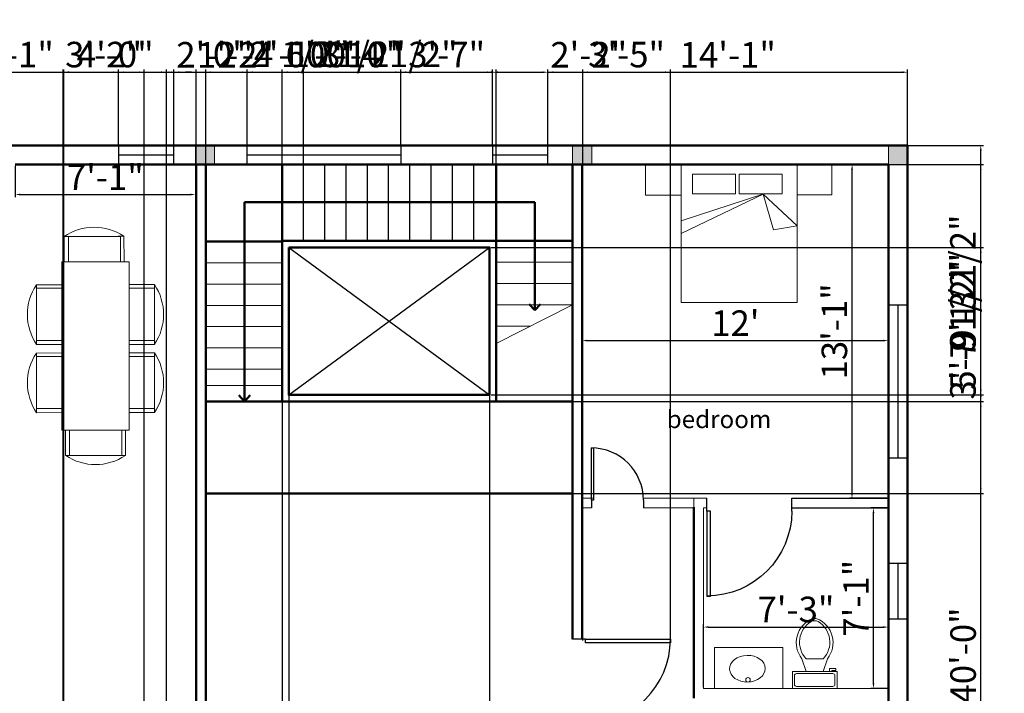
# Model space of a CAD drawing. Units: inches. Extents: x 1367 to 2309, y 1406 to 3826.
# Tile 3 of 9: x 1691 to 2154, y 1853 to 2170. Entities that reach past the tile are written whole.
import ezdxf

# ---------------------------------------------------------------- set-up
doc = ezdxf.new("R2010")
doc.units = ezdxf.units.IN
for name, color, linetype, lineweight in [('A-ANNO-DIMS', 2, 'Continuous', 18), ('A-AREA-IDEN', 3, 'Continuous', 18), ('A-DOOR', 4, 'Continuous', 25), ('A-FLOR-FIXT', 8, 'Continuous', 18), ('A-FLOR-STRS', 7, 'Continuous', 25), ('A-FURN', 8, 'Continuous', 18), ('A-GLAZ', 4, 'Continuous', 25), ('A-WALL', 7, 'Continuous', 50), ('A-WALL-PATT', 8, 'Continuous', 18)]:
    doc.layers.add(name, color=color, linetype=linetype, lineweight=lineweight)
doc.styles.get("Standard").update_dxf_attribs({"font": 'arial.ttf'})
doc.dimstyles.new('ISO-25', dxfattribs={"dimtxt": 12, "dimasz": 2.5, "dimexe": 1.25, "dimexo": 0.625, "dimtad": 1, "dimdec": 0, "dimlunit": 4, "dimtxsty": 'Standard', "dimcen": 2.5, "dimadec": 0, "dimazin": 0, "dimtfac": 1, "dimtdec": 0, "dimtmove": 0, "dimatfit": 3, "dimfxl": 1, "dimarcsym": 0})

# ---------------------------------------------------------------- blocks, each defined once
blk = doc.blocks.new('*U2')
for p, q in [((0, 0), (0, -6)), ((40, 0), (40, -6))]:
    blk.add_line(p, q)
blk.add_lwpolyline([(0, 0), (0, 40), (1.75, 40), (1.75, 0)], close=True)
blk.add_arc((0, 0), 40, 0, 90)
blk = doc.blocks.new('*U4')
for p, q in [((9.5, -6), (9.5, -2)), ((-10, -8.5), (-8, -8.5)), ((-10, -9.5), (-10, -8.5)), ((-8, -8.5), (-8, -8)), ((-7, -8), (-7, -9.5)), ((-4, -8), (-6, -14)), ((4, -8), (6, -14)), ((-7, -9.5), (-10, -9.5)), ((4, -14), (-4, -14))]:
    blk.add_line(p, q)
blk.add_lwpolyline([(10.5, -8), (10.5, 0), (-10.5, 0), (-10.5, -8)], close=True)
for points in [[(-9.5, -2), (-9.5, -6)], [(8.5, -1), (-8.5, -1)], [(-8.5, -7), (8.5, -7)]]:
    blk.add_lwpolyline(points)
for centre, radius, start, end in [((-8.62, -1.88), 0.884, 81.8699, 188.1301), ((8.62, -1.88), 0.884, 351.8699, 98.1301), ((-8.62, -6.12), 0.884, 171.8699, 278.1301), ((8.62, -6.12), 0.884, 261.8699, 8.1301), ((3.52, -21.58), 12.17, 141.4691, 247.9714), ((4.2, -21.82), 11.33, 136.3677, 238.9468), ((-3.52, -21.58), 12.17, 292.0284, 38.5307), ((-4.2, -21.82), 11.33, 301.053, 43.6321), ((0, -27.88), 4, 245.7318, 294.2682), ((0, -29), 4, 254.8605, 285.1395)]:
    blk.add_arc(centre, radius, start, end)
blk = doc.blocks.new('*D27')
at = {"layer": 'A-ANNO-DIMS', "color": 0, "lineweight": -2, "transparency": 16777216}
for p, q in [((1688.87, 2101.5), (1688.87, 2086.74)), ((1773.66, 2101.5), (1773.66, 2086.74)), ((1691.37, 2087.99), (1771.16, 2087.99))]:
    blk.add_line(p, q, dxfattribs=at)
at = {"layer": 'A-ANNO-DIMS', "color": 0, "lineweight": 100, "transparency": 16777216}
for points in [[(1691.37, 2088.41), (1691.37, 2087.58), (1688.87, 2087.99)], [(1771.16, 2088.41), (1771.16, 2087.58), (1773.66, 2087.99)]]:
    blk.add_solid(points, dxfattribs=at)
at = {"layer": 'Defpoints', "color": 0, "lineweight": 100, "transparency": 16777216}
for p in [(1688.87, 2102.13), (1773.66, 2102.13), (1773.66, 2087.99)]:
    blk.add_point(p, dxfattribs=at)
at = {"layer": 'A-ANNO-DIMS', "color": 0, "transparency": 16777216, "insert": (1731.27, 2094.64), "char_height": 12, "attachment_point": 5}
blk.add_mtext('7\'-1"', dxfattribs=at)
blk = doc.blocks.new('*D28')
at = {"layer": 'A-ANNO-DIMS', "color": 0, "lineweight": -2, "transparency": 16777216}
for p, q in [((1955.49, 2101.5), (1955.49, 2018.02)), ((2099.49, 2101.5), (2099.49, 2018.02)), ((1957.99, 2019.27), (2096.99, 2019.27))]:
    blk.add_line(p, q, dxfattribs=at)
at = {"layer": 'A-ANNO-DIMS', "color": 0, "lineweight": 100, "transparency": 16777216}
for points in [[(1957.99, 2019.69), (1957.99, 2018.85), (1955.49, 2019.27)], [(2096.99, 2019.69), (2096.99, 2018.85), (2099.49, 2019.27)]]:
    blk.add_solid(points, dxfattribs=at)
at = {"layer": 'Defpoints', "color": 0, "lineweight": 100, "transparency": 16777216}
for p in [(1955.49, 2102.13), (2099.49, 2102.13), (2099.49, 2019.27)]:
    blk.add_point(p, dxfattribs=at)
at = {"layer": 'A-ANNO-DIMS', "color": 0, "transparency": 16777216, "insert": (2027.49, 2025.92), "char_height": 12, "attachment_point": 5}
blk.add_mtext("12'", dxfattribs=at)
blk = doc.blocks.new('*D29')
at = {"layer": 'A-ANNO-DIMS', "color": 0, "lineweight": -2, "transparency": 16777216}
for p, q in [((2098.9, 2102.13), (2081.16, 2102.13)), ((2082.38, 1947.59), (2082.41, 2099.63)), ((2098.87, 1945.09), (2081.13, 1945.09))]:
    blk.add_line(p, q, dxfattribs=at)
at = {"layer": 'A-ANNO-DIMS', "color": 0, "lineweight": 100, "transparency": 16777216}
for points in [[(2081.99, 2099.63), (2082.83, 2099.63), (2082.41, 2102.13)], [(2081.96, 1947.59), (2082.79, 1947.59), (2082.38, 1945.09)]]:
    blk.add_solid(points, dxfattribs=at)
at = {"layer": 'Defpoints', "color": 0, "lineweight": 100, "transparency": 16777216}
for p in [(2082.41, 2102.13), (2099.53, 2102.13), (2099.49, 1945.09)]:
    blk.add_point(p, dxfattribs=at)
at = {"layer": 'A-ANNO-DIMS', "color": 0, "transparency": 16777216, "insert": (2075.64, 2023.61), "char_height": 12, "attachment_point": 5, "rotation": 89.9877}
blk.add_mtext('13\'-1"', dxfattribs=at)
blk = doc.blocks.new('*D30')
at = {"layer": 'A-ANNO-DIMS', "color": 0, "lineweight": -2, "transparency": 16777216}
for p, q in [((2098.87, 1940.59), (2091.22, 1940.59)), ((2092.47, 1858.08), (2092.47, 1938.09)), ((2098.87, 1855.58), (2091.22, 1855.58))]:
    blk.add_line(p, q, dxfattribs=at)
at = {"layer": 'A-ANNO-DIMS', "color": 0, "lineweight": 100, "transparency": 16777216}
for points in [[(2092.05, 1938.09), (2092.89, 1938.09), (2092.47, 1940.59)], [(2092.05, 1858.08), (2092.89, 1858.08), (2092.47, 1855.58)]]:
    blk.add_solid(points, dxfattribs=at)
at = {"layer": 'Defpoints', "color": 0, "lineweight": 100, "transparency": 16777216}
for p in [(2092.47, 1940.59), (2099.49, 1940.59), (2099.49, 1855.58)]:
    blk.add_point(p, dxfattribs=at)
at = {"layer": 'A-ANNO-DIMS', "color": 0, "transparency": 16777216, "insert": (2085.82, 1898.08), "char_height": 12, "attachment_point": 5, "rotation": 90}
blk.add_mtext('7\'-1"', dxfattribs=at)
blk = doc.blocks.new('*D31')
at = {"layer": 'A-ANNO-DIMS', "color": 0, "lineweight": -2, "transparency": 16777216}
for p, q in [((2012.53, 1856.2), (2012.53, 1885.73)), ((2015.03, 1884.48), (2096.99, 1884.48)), ((2099.49, 1856.2), (2099.49, 1885.73))]:
    blk.add_line(p, q, dxfattribs=at)
at = {"layer": 'A-ANNO-DIMS', "color": 0, "lineweight": 100, "transparency": 16777216}
for points in [[(2015.03, 1884.9), (2015.03, 1884.07), (2012.53, 1884.48)], [(2096.99, 1884.9), (2096.99, 1884.07), (2099.49, 1884.48)]]:
    blk.add_solid(points, dxfattribs=at)
at = {"layer": 'Defpoints', "color": 0, "lineweight": 100, "transparency": 16777216}
for p in [(2099.49, 1884.48), (2012.53, 1855.58), (2099.49, 1855.58)]:
    blk.add_point(p, dxfattribs=at)
at = {"layer": 'A-ANNO-DIMS', "color": 0, "transparency": 16777216, "insert": (2056.01, 1891.24), "char_height": 12, "attachment_point": 5}
blk.add_mtext('7\'-3"', dxfattribs=at)
blk = doc.blocks.new('CHAIR')
for p, q in [((0, 28.09), (11.92, 28.09)), ((11.92, 28.09), (11.92, 24.96)), ((0, 0), (11.92, 0)), ((11.92, 0), (11.92, 2.65))]:
    blk.add_line(p, q)
blk.add_arc((-8.81, 14.05), 25.04, 325.887, 34.113)
blk = doc.blocks.new('*D60')
at = {"layer": 'A-ANNO-DIMS', "color": 0, "lineweight": -2, "transparency": 16777216}
for p, q in [((1640.53, 2111.75), (1640.53, 2146.78)), ((1643.03, 2145.53), (1734.96, 2145.53)), ((1737.46, 2111.75), (1737.46, 2146.78))]:
    blk.add_line(p, q, dxfattribs=at)
at = {"layer": 'A-ANNO-DIMS', "color": 0, "lineweight": 100, "transparency": 16777216}
for points in [[(1643.03, 2145.94), (1643.03, 2145.11), (1640.53, 2145.53)], [(1734.96, 2145.94), (1734.96, 2145.11), (1737.46, 2145.53)]]:
    blk.add_solid(points, dxfattribs=at)
at = {"layer": 'Defpoints', "color": 0, "lineweight": 100, "transparency": 16777216}
for p in [(1737.46, 2145.53), (1640.53, 2111.13), (1737.46, 2111.13)]:
    blk.add_point(p, dxfattribs=at)
at = {"layer": 'A-ANNO-DIMS', "color": 0, "transparency": 16777216, "insert": (1688.99, 2152.28), "char_height": 12, "attachment_point": 5}
blk.add_mtext('8\'-1"', dxfattribs=at)
blk = doc.blocks.new('*D61')
at = {"layer": 'A-ANNO-DIMS', "color": 0, "lineweight": -2, "transparency": 16777216}
for p, q in [((1737.46, 2111.75), (1737.46, 2146.78)), ((1739.96, 2145.53), (1761.02, 2145.53)), ((1763.52, 2111.75), (1763.52, 2146.78)), ((1763.52, 2145.53), (1799.38, 2145.53))]:
    blk.add_line(p, q, dxfattribs=at)
at = {"layer": 'A-ANNO-DIMS', "color": 0, "lineweight": 100, "transparency": 16777216}
for points in [[(1739.96, 2145.94), (1739.96, 2145.11), (1737.46, 2145.53)], [(1761.02, 2145.94), (1761.02, 2145.11), (1763.52, 2145.53)]]:
    blk.add_solid(points, dxfattribs=at)
at = {"layer": 'Defpoints', "color": 0, "lineweight": 100, "transparency": 16777216}
for p in [(1763.52, 2145.53), (1737.46, 2111.13), (1763.52, 2111.13)]:
    blk.add_point(p, dxfattribs=at)
at = {"layer": 'A-ANNO-DIMS', "color": 0, "transparency": 16777216, "insert": (1782.7, 2152.18), "char_height": 12, "attachment_point": 5}
blk.add_mtext('2\'-2"', dxfattribs=at)
blk = doc.blocks.new('*D62')
at = {"layer": 'A-ANNO-DIMS', "color": 0, "lineweight": -2, "transparency": 16777216}
for p, q in [((1763.52, 2111.75), (1763.52, 2146.78)), ((1766.02, 2145.53), (1795.49, 2145.53)), ((1797.99, 2111.75), (1797.99, 2146.78)), ((1797.99, 2145.53), (1871.13, 2145.53))]:
    blk.add_line(p, q, dxfattribs=at)
at = {"layer": 'A-ANNO-DIMS', "color": 0, "lineweight": 100, "transparency": 16777216}
for points in [[(1766.02, 2145.94), (1766.02, 2145.11), (1763.52, 2145.53)], [(1795.49, 2145.94), (1795.49, 2145.11), (1797.99, 2145.53)]]:
    blk.add_solid(points, dxfattribs=at)
at = {"layer": 'Defpoints', "color": 0, "lineweight": 100, "transparency": 16777216}
for p in [(1797.99, 2145.53), (1763.52, 2111.13), (1797.99, 2111.13)]:
    blk.add_point(p, dxfattribs=at)
at = {"layer": 'A-ANNO-DIMS', "color": 0, "transparency": 16777216, "insert": (1835.81, 2152.36), "char_height": 12, "attachment_point": 5}
blk.add_mtext('2\'-10 1/2"', dxfattribs=at)
blk = doc.blocks.new('*D63')
at = {"layer": 'A-ANNO-DIMS', "color": 0, "lineweight": -2, "transparency": 16777216}
for p, q in [((1797.99, 2111.75), (1797.99, 2146.78)), ((1800.49, 2145.53), (1867.65, 2145.53)), ((1870.15, 2111.75), (1870.15, 2146.78))]:
    blk.add_line(p, q, dxfattribs=at)
at = {"layer": 'A-ANNO-DIMS', "color": 0, "lineweight": 100, "transparency": 16777216}
for points in [[(1800.49, 2145.94), (1800.49, 2145.11), (1797.99, 2145.53)], [(1867.65, 2145.94), (1867.65, 2145.11), (1870.15, 2145.53)]]:
    blk.add_solid(points, dxfattribs=at)
at = {"layer": 'Defpoints', "color": 0, "lineweight": 100, "transparency": 16777216}
for p in [(1870.15, 2145.53), (1797.99, 2111.13), (1870.15, 2111.13)]:
    blk.add_point(p, dxfattribs=at)
at = {"layer": 'A-ANNO-DIMS', "color": 0, "transparency": 16777216, "insert": (1834.07, 2152.28), "char_height": 12, "attachment_point": 5}
blk.add_mtext('6\'-0"', dxfattribs=at)
blk = doc.blocks.new('*D64')
at = {"layer": 'A-ANNO-DIMS', "color": 0, "lineweight": -2, "transparency": 16777216}
for p, q in [((1870.15, 2111.75), (1870.15, 2146.78)), ((1872.65, 2145.53), (1910.84, 2145.53)), ((1913.34, 2111.75), (1913.34, 2146.78))]:
    blk.add_line(p, q, dxfattribs=at)
at = {"layer": 'A-ANNO-DIMS', "color": 0, "lineweight": 100, "transparency": 16777216}
for points in [[(1872.65, 2145.94), (1872.65, 2145.11), (1870.15, 2145.53)], [(1910.84, 2145.94), (1910.84, 2145.11), (1913.34, 2145.53)]]:
    blk.add_solid(points, dxfattribs=at)
at = {"layer": 'Defpoints', "color": 0, "lineweight": 100, "transparency": 16777216}
for p in [(1913.34, 2145.53), (1870.15, 2111.13), (1913.34, 2111.13)]:
    blk.add_point(p, dxfattribs=at)
at = {"layer": 'A-ANNO-DIMS', "color": 0, "transparency": 16777216, "insert": (1891.75, 2152.28), "char_height": 12, "attachment_point": 5}
blk.add_mtext('3\'-7"', dxfattribs=at)
blk = doc.blocks.new('*D65')
at = {"layer": 'A-ANNO-DIMS', "color": 0, "lineweight": -2, "transparency": 16777216}
for p, q in [((1913.34, 2111.75), (1913.34, 2146.78)), ((1915.84, 2145.53), (1936.9, 2145.53)), ((1939.4, 2111.75), (1939.4, 2146.78)), ((1939.4, 2145.53), (1975.25, 2145.53))]:
    blk.add_line(p, q, dxfattribs=at)
at = {"layer": 'A-ANNO-DIMS', "color": 0, "lineweight": 100, "transparency": 16777216}
for points in [[(1915.84, 2145.94), (1915.84, 2145.11), (1913.34, 2145.53)], [(1936.9, 2145.94), (1936.9, 2145.11), (1939.4, 2145.53)]]:
    blk.add_solid(points, dxfattribs=at)
at = {"layer": 'Defpoints', "color": 0, "lineweight": 100, "transparency": 16777216}
for p in [(1939.4, 2145.53), (1913.34, 2111.13), (1939.4, 2111.13)]:
    blk.add_point(p, dxfattribs=at)
at = {"layer": 'A-ANNO-DIMS', "color": 0, "transparency": 16777216, "insert": (1958.58, 2152.18), "char_height": 12, "attachment_point": 5}
blk.add_mtext('2\'-2"', dxfattribs=at)
blk = doc.blocks.new('*D66')
at = {"layer": 'A-ANNO-DIMS', "color": 0, "lineweight": -2, "transparency": 16777216}
for p, q in [((1939.4, 2111.75), (1939.4, 2146.78)), ((1941.9, 2145.53), (2106.03, 2145.53)), ((2108.53, 2111.75), (2108.53, 2146.78))]:
    blk.add_line(p, q, dxfattribs=at)
at = {"layer": 'A-ANNO-DIMS', "color": 0, "lineweight": 100, "transparency": 16777216}
for points in [[(1941.9, 2145.94), (1941.9, 2145.11), (1939.4, 2145.53)], [(2106.03, 2145.94), (2106.03, 2145.11), (2108.53, 2145.53)]]:
    blk.add_solid(points, dxfattribs=at)
at = {"layer": 'Defpoints', "color": 0, "lineweight": 100, "transparency": 16777216}
for p in [(2108.53, 2145.53), (1939.4, 2111.13), (2108.53, 2111.13)]:
    blk.add_point(p, dxfattribs=at)
at = {"layer": 'A-ANNO-DIMS', "color": 0, "transparency": 16777216, "insert": (2023.96, 2152.18), "char_height": 12, "attachment_point": 5}
blk.add_mtext('14\'-1"', dxfattribs=at)
blk = doc.blocks.new('*D67')
at = {"layer": 'A-ANNO-DIMS', "color": 0, "lineweight": -2, "transparency": 16777216}
for p, q in [((2109.15, 2111.13), (2144.18, 2111.13)), ((2142.93, 1633.63), (2142.93, 2108.63)), ((2109.12, 1631.13), (2144.18, 1631.13))]:
    blk.add_line(p, q, dxfattribs=at)
at = {"layer": 'A-ANNO-DIMS', "color": 0, "lineweight": 100, "transparency": 16777216}
for points in [[(2142.51, 2108.63), (2143.34, 2108.63), (2142.93, 2111.13)], [(2142.51, 1633.63), (2143.34, 1633.63), (2142.93, 1631.13)]]:
    blk.add_solid(points, dxfattribs=at)
at = {"layer": 'Defpoints', "color": 0, "lineweight": 100, "transparency": 16777216}
for p in [(2108.53, 2111.13), (2142.93, 2111.13), (2108.49, 1631.13)]:
    blk.add_point(p, dxfattribs=at)
at = {"layer": 'A-ANNO-DIMS', "color": 0, "transparency": 16777216, "insert": (2136.17, 1871.13), "char_height": 12, "attachment_point": 5, "rotation": 90}
blk.add_mtext('40\'-0"', dxfattribs=at)
blk = doc.blocks.new('*D76')
at = {"layer": 'A-ANNO-DIMS', "color": 0, "lineweight": -2, "transparency": 16777216}
for p, q in [((1711.82, 1517.28), (1711.82, 2146.78)), ((1714.32, 2145.53), (1757.51, 2145.53)), ((1760.01, 1517.28), (1760.01, 2146.78))]:
    blk.add_line(p, q, dxfattribs=at)
at = {"layer": 'A-ANNO-DIMS', "color": 0, "lineweight": 100, "transparency": 16777216}
for points in [[(1714.32, 2145.94), (1714.32, 2145.11), (1711.82, 2145.53)], [(1757.51, 2145.94), (1757.51, 2145.11), (1760.01, 2145.53)]]:
    blk.add_solid(points, dxfattribs=at)
at = {"layer": 'Defpoints', "color": 0, "lineweight": 100, "transparency": 16777216}
for p in [(1760.01, 2145.53), (1711.82, 1516.65), (1760.01, 1516.65)]:
    blk.add_point(p, dxfattribs=at)
at = {"layer": 'A-ANNO-DIMS', "color": 0, "transparency": 16777216, "insert": (1735.92, 2152.28), "char_height": 12, "attachment_point": 5}
blk.add_mtext('4\'-0"', dxfattribs=at)
blk = doc.blocks.new('*D77')
at = {"layer": 'A-ANNO-DIMS', "color": 0, "lineweight": -2, "transparency": 16777216}
for p, q in [((1760.01, 1493.18), (1760.01, 2146.78)), ((1762.51, 2145.53), (1771.49, 2145.53)), ((1773.99, 1493.56), (1773.99, 2146.78)), ((1773.99, 2145.53), (1808.51, 2145.53))]:
    blk.add_line(p, q, dxfattribs=at)
at = {"layer": 'A-ANNO-DIMS', "color": 0, "lineweight": 100, "transparency": 16777216}
for points in [[(1762.51, 2145.94), (1762.51, 2145.11), (1760.01, 2145.53)], [(1771.49, 2145.94), (1771.49, 2145.11), (1773.99, 2145.53)]]:
    blk.add_solid(points, dxfattribs=at)
at = {"layer": 'Defpoints', "color": 0, "lineweight": 100, "transparency": 16777216}
for p in [(1773.99, 2145.53), (1760.01, 1492.55), (1773.99, 1492.94)]:
    blk.add_point(p, dxfattribs=at)
at = {"layer": 'A-ANNO-DIMS', "color": 0, "transparency": 16777216, "insert": (1792.5, 2152.18), "char_height": 12, "attachment_point": 5}
blk.add_mtext('1\'-2"', dxfattribs=at)
blk = doc.blocks.new('*D78')
at = {"layer": 'A-ANNO-DIMS', "color": 0, "lineweight": -2, "transparency": 16777216}
for p, q in [((1711.4, 1640.75), (1711.4, 2146.78)), ((1713.9, 2145.53), (1747.03, 2145.53)), ((1749.53, 1640.75), (1749.53, 2146.78))]:
    blk.add_line(p, q, dxfattribs=at)
at = {"layer": 'A-ANNO-DIMS', "color": 0, "lineweight": 100, "transparency": 16777216}
for points in [[(1713.9, 2145.94), (1713.9, 2145.11), (1711.4, 2145.53)], [(1747.03, 2145.94), (1747.03, 2145.11), (1749.53, 2145.53)]]:
    blk.add_solid(points, dxfattribs=at)
at = {"layer": 'Defpoints', "color": 0, "lineweight": 100, "transparency": 16777216}
for p in [(1749.53, 2145.53), (1711.4, 1640.13), (1749.53, 1640.13)]:
    blk.add_point(p, dxfattribs=at)
at = {"layer": 'A-ANNO-DIMS', "color": 0, "transparency": 16777216, "insert": (1730.47, 2152.28), "char_height": 12, "attachment_point": 5}
blk.add_mtext('3\'-2"', dxfattribs=at)
blk = doc.blocks.new('*D79')
at = {"layer": 'A-ANNO-DIMS', "color": 0, "lineweight": -2, "transparency": 16777216}
for p, q in [((1778.49, 1990.06), (1778.49, 1415.33)), ((1814.49, 1990.06), (1814.49, 1415.33)), ((1780.99, 1416.58), (1811.99, 1416.58))]:
    blk.add_line(p, q, dxfattribs=at)
at = {"layer": 'A-ANNO-DIMS', "color": 0, "lineweight": 100, "transparency": 16777216}
for points in [[(1780.99, 1416.99), (1780.99, 1416.16), (1778.49, 1416.58)], [(1811.99, 1416.99), (1811.99, 1416.16), (1814.49, 1416.58)]]:
    blk.add_solid(points, dxfattribs=at)
at = {"layer": 'Defpoints', "color": 0, "lineweight": 100, "transparency": 16777216}
for p in [(1778.49, 1990.68), (1814.49, 1990.68), (1814.49, 1416.58)]:
    blk.add_point(p, dxfattribs=at)
at = {"layer": 'A-ANNO-DIMS', "color": 0, "transparency": 16777216, "insert": (1796.49, 1423.33), "char_height": 12, "attachment_point": 5}
blk.add_mtext('3\'-0"', dxfattribs=at)
blk = doc.blocks.new('*D80')
at = {"layer": 'A-ANNO-DIMS', "color": 0, "lineweight": -2, "transparency": 16777216}
for p, q in [((1817.49, 1993.06), (1817.49, 1415.33)), ((1911.99, 1993.06), (1911.99, 1415.33)), ((1819.99, 1416.58), (1909.49, 1416.58))]:
    blk.add_line(p, q, dxfattribs=at)
at = {"layer": 'A-ANNO-DIMS', "color": 0, "lineweight": 100, "transparency": 16777216}
for points in [[(1819.99, 1416.99), (1819.99, 1416.16), (1817.49, 1416.58)], [(1909.49, 1416.99), (1909.49, 1416.16), (1911.99, 1416.58)]]:
    blk.add_solid(points, dxfattribs=at)
at = {"layer": 'Defpoints', "color": 0, "lineweight": 100, "transparency": 16777216}
for p in [(1817.49, 1993.68), (1911.99, 1993.68), (1911.99, 1416.58)]:
    blk.add_point(p, dxfattribs=at)
at = {"layer": 'A-ANNO-DIMS', "color": 0, "transparency": 16777216, "insert": (1864.74, 1423.41), "char_height": 12, "attachment_point": 5}
blk.add_mtext('7\'-10 1/2"', dxfattribs=at)
blk = doc.blocks.new('*D81')
at = {"layer": 'A-ANNO-DIMS', "color": 0, "lineweight": -2, "transparency": 16777216}
for p, q in [((1912.62, 2063.13), (2144.18, 2063.13)), ((2142.93, 1996.18), (2142.93, 2060.63)), ((1912.62, 1993.68), (2144.18, 1993.68))]:
    blk.add_line(p, q, dxfattribs=at)
at = {"layer": 'A-ANNO-DIMS', "color": 0, "lineweight": 100, "transparency": 16777216}
for points in [[(2142.51, 2060.63), (2143.34, 2060.63), (2142.93, 2063.13)], [(2142.51, 1996.18), (2143.34, 1996.18), (2142.93, 1993.68)]]:
    blk.add_solid(points, dxfattribs=at)
at = {"layer": 'Defpoints', "color": 0, "lineweight": 100, "transparency": 16777216}
for p in [(1911.99, 2063.13), (2142.93, 2063.13), (1911.99, 1993.68)]:
    blk.add_point(p, dxfattribs=at)
at = {"layer": 'A-ANNO-DIMS', "color": 0, "transparency": 16777216, "insert": (2136.1, 2028.41), "char_height": 12, "attachment_point": 5, "rotation": 90}
blk.add_mtext('5\'-9 1/2"', dxfattribs=at)
blk = doc.blocks.new('*D82')
at = {"layer": 'A-ANNO-DIMS', "color": 0, "lineweight": -2, "transparency": 16777216}
for p, q in [((1814.49, 2066.46), (1814.49, 2146.78)), ((1816.99, 2145.53), (1912.49, 2145.53)), ((1914.99, 2066.75), (1914.99, 2146.78))]:
    blk.add_line(p, q, dxfattribs=at)
at = {"layer": 'A-ANNO-DIMS', "color": 0, "lineweight": 100, "transparency": 16777216}
for points in [[(1816.99, 2145.94), (1816.99, 2145.11), (1814.49, 2145.53)], [(1912.49, 2145.94), (1912.49, 2145.11), (1914.99, 2145.53)]]:
    blk.add_solid(points, dxfattribs=at)
at = {"layer": 'Defpoints', "color": 0, "lineweight": 100, "transparency": 16777216}
for p in [(1914.99, 2145.53), (1814.49, 2065.83), (1914.99, 2066.13)]:
    blk.add_point(p, dxfattribs=at)
at = {"layer": 'A-ANNO-DIMS', "color": 0, "transparency": 16777216, "insert": (1864.74, 2152.36), "char_height": 12, "attachment_point": 5}
blk.add_mtext('8\'-4 1/2"', dxfattribs=at)
blk = doc.blocks.new('*D83')
at = {"layer": 'A-ANNO-DIMS', "color": 0, "lineweight": -2, "transparency": 16777216}
for p, q in [((1814.49, 2066.46), (1814.49, 2146.78)), ((1816.99, 2145.53), (1821.99, 2145.53)), ((1824.49, 2066.46), (1824.49, 2146.78)), ((1824.49, 2145.53), (1869.47, 2145.53))]:
    blk.add_line(p, q, dxfattribs=at)
at = {"layer": 'A-ANNO-DIMS', "color": 0, "lineweight": 100, "transparency": 16777216}
for points in [[(1816.99, 2145.94), (1816.99, 2145.11), (1814.49, 2145.53)], [(1821.99, 2145.94), (1821.99, 2145.11), (1824.49, 2145.53)]]:
    blk.add_solid(points, dxfattribs=at)
at = {"layer": 'Defpoints', "color": 0, "lineweight": 100, "transparency": 16777216}
for p in [(1824.49, 2145.53), (1814.49, 2065.83), (1824.49, 2065.83)]:
    blk.add_point(p, dxfattribs=at)
at = {"layer": 'A-ANNO-DIMS', "color": 0, "transparency": 16777216, "insert": (1848.23, 2152.28), "char_height": 12, "attachment_point": 5}
blk.add_mtext('0\'-10"', dxfattribs=at)
blk = doc.blocks.new('*D84')
at = {"layer": 'A-ANNO-DIMS', "color": 0, "lineweight": -2, "transparency": 16777216}
for p, q in [((2142.93, 1990.68), (2142.93, 2054.29)), ((1951.62, 1990.68), (2144.18, 1990.68)), ((2142.93, 1949.83), (2142.93, 1988.18)), ((1951.62, 1947.33), (2144.18, 1947.33))]:
    blk.add_line(p, q, dxfattribs=at)
at = {"layer": 'A-ANNO-DIMS', "color": 0, "lineweight": 100, "transparency": 16777216}
for points in [[(2142.51, 1988.18), (2143.34, 1988.18), (2142.93, 1990.68)], [(2142.51, 1949.83), (2143.34, 1949.83), (2142.93, 1947.33)]]:
    blk.add_solid(points, dxfattribs=at)
at = {"layer": 'Defpoints', "color": 0, "lineweight": 100, "transparency": 16777216}
for p in [(1950.99, 1990.68), (2142.93, 1990.68), (1950.99, 1947.33)]:
    blk.add_point(p, dxfattribs=at)
at = {"layer": 'A-ANNO-DIMS', "color": 0, "transparency": 16777216, "insert": (2136.09, 2023.73), "char_height": 12, "attachment_point": 5, "rotation": 90}
blk.add_mtext('3\'-7 1/2"', dxfattribs=at)
blk = doc.blocks.new('*D85')
at = {"layer": 'A-ANNO-DIMS', "color": 0, "lineweight": -2, "transparency": 16777216}
for p, q in [((1951.62, 2102.13), (2144.18, 2102.13)), ((2142.93, 1993.18), (2142.93, 2099.63)), ((1951.62, 1990.68), (2144.18, 1990.68))]:
    blk.add_line(p, q, dxfattribs=at)
at = {"layer": 'A-ANNO-DIMS', "color": 0, "lineweight": 100, "transparency": 16777216}
for points in [[(2142.51, 2099.63), (2143.34, 2099.63), (2142.93, 2102.13)], [(2142.51, 1993.18), (2143.34, 1993.18), (2142.93, 1990.68)]]:
    blk.add_solid(points, dxfattribs=at)
at = {"layer": 'Defpoints', "color": 0, "lineweight": 100, "transparency": 16777216}
for p in [(1950.99, 2102.13), (2142.93, 2102.13), (1950.99, 1990.68)]:
    blk.add_point(p, dxfattribs=at)
at = {"layer": 'A-ANNO-DIMS', "color": 0, "transparency": 16777216, "insert": (2136.09, 2046.41), "char_height": 12, "attachment_point": 5, "rotation": 90}
blk.add_mtext('9\'-3 1/2"', dxfattribs=at)
blk = doc.blocks.new('*D86')
at = {"layer": 'A-ANNO-DIMS', "color": 0, "lineweight": -2, "transparency": 16777216}
for p, q in [((1771.49, 2145.53), (1768.99, 2145.53)), ((1773.99, 2102.75), (1773.99, 2146.78)), ((1773.99, 2145.53), (1778.49, 2145.53)), ((1778.49, 2102.75), (1778.49, 2146.78)), ((1780.99, 2145.53), (1844.6, 2145.53))]:
    blk.add_line(p, q, dxfattribs=at)
at = {"layer": 'A-ANNO-DIMS', "color": 0, "lineweight": 100, "transparency": 16777216}
for points in [[(1771.49, 2145.94), (1771.49, 2145.11), (1773.99, 2145.53)], [(1780.99, 2145.94), (1780.99, 2145.11), (1778.49, 2145.53)]]:
    blk.add_solid(points, dxfattribs=at)
at = {"layer": 'Defpoints', "color": 0, "lineweight": 100, "transparency": 16777216}
for p in [(1778.49, 2145.53), (1773.99, 2102.13), (1778.49, 2102.13)]:
    blk.add_point(p, dxfattribs=at)
at = {"layer": 'A-ANNO-DIMS', "color": 0, "transparency": 16777216, "insert": (1814.05, 2152.36), "char_height": 12, "attachment_point": 5}
blk.add_mtext('0\'-4 1/2"', dxfattribs=at)
blk = doc.blocks.new('*D137')
at = {"layer": 'A-ANNO-DIMS', "color": 0, "lineweight": -2, "transparency": 16777216}
for p, q in [((1955.76, 1878.24), (1955.76, 2146.78)), ((1958.26, 2145.53), (1994.49, 2145.53)), ((1996.99, 1877.73), (1996.99, 2146.78))]:
    blk.add_line(p, q, dxfattribs=at)
at = {"layer": 'A-ANNO-DIMS', "color": 0, "lineweight": 100, "transparency": 16777216}
for points in [[(1958.26, 2145.94), (1958.26, 2145.11), (1955.76, 2145.53)], [(1994.49, 2145.94), (1994.49, 2145.11), (1996.99, 2145.53)]]:
    blk.add_solid(points, dxfattribs=at)
at = {"layer": 'Defpoints', "color": 0, "lineweight": 100, "transparency": 16777216}
for p in [(1996.99, 2145.53), (1955.76, 1877.62), (1996.99, 1877.1)]:
    blk.add_point(p, dxfattribs=at)
at = {"layer": 'A-ANNO-DIMS', "color": 0, "transparency": 16777216, "insert": (1976.37, 2152.28), "char_height": 12, "attachment_point": 5}
blk.add_mtext('3\'-5"', dxfattribs=at)

msp = doc.modelspace()

# ---------------------------------------------------------------- hatches: boundary and pattern name
at = {"layer": 'A-WALL-PATT'}
h = msp.add_hatch(color=256, dxfattribs=at)
h.dxf.hatch_style = 1
h.paths.add_polyline_path([(2108.49, 2102.13), (2108.49, 2111.13), (2099.53, 2111.13), (2099.53, 2102.13)])
h.paths.add_polyline_path([(1959.99, 2102.13), (1959.99, 2111.13), (1950.99, 2111.13), (1950.99, 2102.13)])
h.paths.add_polyline_path([(1773.66, 2111.13), (1773.66, 2102.13), (1782.66, 2102.13), (1782.66, 2111.13)])
h = msp.add_hatch(color=256, dxfattribs=at)
h.dxf.hatch_style = 1
h.paths.add_polyline_path([(1508.49, 1631.13), (1517.49, 1631.13), (1517.49, 1640.13), (1508.49, 1640.13)])
h.paths.add_polyline_path([(1773.99, 1631.13), (1782.99, 1631.13), (1782.99, 1640.13), (1773.99, 1640.13)])
h.paths.add_polyline_path([(1959.99, 1631.13), (1959.99, 1640.13), (1950.99, 1640.13), (1950.99, 1631.13)])
h.paths.add_polyline_path([(2099.49, 1640.13), (2099.49, 1631.13), (2108.49, 1631.13), (2108.49, 1640.13)])
h.paths.add_polyline_path([(1706.06, 1795.81), (1771.22, 1795.81), (1771.22, 1813.02), (1706.06, 1813.02)], flags=9)
h.paths.add_polyline_path([(1573.51, 1725.43), (1623.74, 1725.43), (1623.74, 1742.65), (1573.51, 1742.65)], flags=9)
h.paths.add_polyline_path([(1582.26, 2004.3), (1623.41, 2004.3), (1623.41, 2021.52), (1582.26, 2021.52)], flags=9)
h.paths.add_polyline_path([(1992.39, 1973.53), (2042.62, 1973.53), (2042.62, 1990.75), (1992.39, 1990.75)], flags=9)
h.paths.add_polyline_path([(2015.09, 1737.31), (2065.32, 1737.31), (2065.32, 1754.53), (2015.09, 1754.53)], flags=9)
h.paths.add_polyline_path([(1827.45, 1770.85), (1884.81, 1770.85), (1884.81, 1788.06), (1827.45, 1788.06)], flags=9)

# ---------------------------------------------------------------- linework, layer by layer
at = {"layer": 'A-FLOR-STRS'}
for p, q in [((1824.49, 2065.83), (1824.49, 2102.13)), ((1834.49, 2065.83), (1834.49, 2102.13)), ((1844.49, 2065.83), (1844.49, 2102.13)), ((1854.49, 2065.83), (1854.49, 2102.13)), ((1864.49, 2065.83), (1864.49, 2102.13)), ((1874.49, 2065.83), (1874.49, 2102.13)), ((1884.49, 2065.83), (1884.49, 2102.13)), ((1894.49, 2065.83), (1894.49, 2102.13)), ((1904.49, 2065.83), (1904.49, 2102.13)), ((1817.49, 2063.13), (1911.99, 1993.68)), ((1817.49, 1993.68), (1911.99, 2063.13))]:
    msp.add_line(p, q, dxfattribs=at)
at = {"layer": 'A-FURN'}
for p, q in [((2040.89, 2088.29), (2002.08, 2075.58)), ((2040.89, 2088.29), (2002.08, 2069.66)), ((2040.56, 2088.13), (2056.63, 2073.27)), ((2045.41, 2071.32), (2040.56, 2088.13)), ((2056.63, 2073.27), (2045.41, 2071.32)), ((1778.49, 2055.83), (1814.49, 2055.83)), ((1914.99, 2056.13), (1950.99, 2056.13)), ((1778.49, 2045.83), (1814.49, 2045.83)), ((1914.99, 2046.13), (1950.99, 2046.13)), ((1778.49, 2035.83), (1814.49, 2035.83)), ((1914.99, 2036.13), (1950.99, 2036.13)), ((1914.99, 2017.94), (1950.99, 2036.13)), ((1778.49, 2025.83), (1814.49, 2025.83)), ((1914.99, 2026.13), (1931.19, 2026.13)), ((1778.49, 2015.83), (1814.49, 2015.83)), ((1778.49, 2005.83), (1814.49, 2005.83)), ((1778.49, 1998.12), (1814.49, 1998.12)), ((1960.87, 1945.09), (1955.49, 1945.09)), ((2008.03, 1945.09), (1984.28, 1945.09)), ((2008.03, 1945.09), (2014.06, 1945.09)), ((2008.03, 1940.59), (2008.03, 1945.09)), ((1959.8, 1940.59), (1955.49, 1940.59)), ((2008.03, 1940.59), (1984.29, 1940.59)), ((2004.29, 1940.59), (2008.03, 1940.59)), ((2012.53, 1940.59), (2014.06, 1940.59)), ((2012.53, 1940.59), (2012.53, 1855.58)), ((2017.75, 1855.58), (2017.75, 1874.93)), ((2096.58, 1855.58), (2012.53, 1855.58)), ((2012.53, 1855.58), (2099.49, 1855.58)), ((2096.58, 1855.58), (2099.49, 1855.58))]:
    msp.add_line(p, q, dxfattribs=at)
for points in [[(1773.66, 2111.13), (1782.66, 2111.13), (1782.66, 2102.13), (1773.66, 2102.13)], [(1950.99, 2111.13), (1959.99, 2111.13), (1959.99, 2102.13), (1950.99, 2102.13)], [(2099.53, 2111.13), (2108.53, 2111.13), (2108.53, 2102.13), (2099.53, 2102.13)], [(2002.08, 2102.13), (1985.26, 2102.13), (1985.26, 2087.72), (2002.08, 2087.72)], [(2002.08, 2102.13), (2056.63, 2102.13), (2056.63, 2037.19), (2002.08, 2037.19)], [(2056.63, 2102.13), (2072.9, 2102.13), (2072.9, 2087.87), (2056.63, 2087.87)], [(2007.44, 2097.5), (2027.64, 2097.5), (2027.64, 2088.29), (2007.44, 2088.29)], [(2029.32, 2097.5), (2049.51, 2097.5), (2049.51, 2088.29), (2029.32, 2088.29)], [(1738.42, 2056.37), (1738.42, 2068.29), (1713.9, 2068.29), (1713.9, 2056.37)], [(1710.82, 2056.37), (1742.44, 2056.37), (1742.44, 1977.17), (1710.82, 1977.17)], [(1710.82, 2043.91), (1698.9, 2043.91), (1698.9, 2019.39), (1710.82, 2019.39)], [(1742.44, 2043.91), (1754.36, 2043.91), (1754.36, 2019.39), (1742.44, 2019.39)], [(1710.82, 2011.81), (1698.9, 2011.81), (1698.9, 1987.3), (1710.82, 1987.3)], [(1742.44, 2011.81), (1754.36, 2011.81), (1754.36, 1987.3), (1742.44, 1987.3)], [(1739.01, 1977.17), (1739.01, 1965.25), (1714.49, 1965.25), (1714.49, 1977.17)], [(2017.75, 1874.93), (2017.75, 1855.58), (2049.92, 1855.58), (2049.92, 1874.93)]]:
    msp.add_lwpolyline(points, close=True, dxfattribs=at)
msp.add_circle((2033.44, 1859.68), 1.06, dxfattribs=at)
msp.add_ellipse((2033.19, 1864.89), major_axis=(8.38, 0.17), ratio=0.747916, dxfattribs=at)
at = {"layer": 'A-GLAZ'}
for p, q in [((1737.46, 2106.63), (1763.52, 2106.63)), ((1797.99, 2106.63), (1870.15, 2106.63)), ((1913.34, 2106.63), (1939.4, 2106.63)), ((2103.99, 2036.08), (2103.99, 1963.92)), ((2054.06, 1945.09), (2099.49, 1945.09)), ((2054.06, 1940.59), (2099.49, 1940.59)), ((2103.99, 1914.39), (2103.99, 1888.32))]:
    msp.add_line(p, q, dxfattribs=at)
for points in [[(1737.46, 2102.13), (1763.52, 2102.13), (1763.52, 2111.13), (1737.46, 2111.13)], [(1797.99, 2111.13), (1870.15, 2111.13), (1870.15, 2102.13), (1797.99, 2102.13)], [(1913.34, 2102.13), (1939.4, 2102.13), (1939.4, 2111.13), (1913.34, 2111.13)], [(2108.49, 2036.08), (2108.49, 1963.92), (2099.49, 1963.92), (2099.49, 2036.08)], [(2099.49, 1914.39), (2099.49, 1888.32), (2108.49, 1888.32), (2108.49, 1914.39)]]:
    msp.add_lwpolyline(points, close=True, dxfattribs=at)
at = {"layer": 'A-WALL'}
for p, q in [((1688.87, 2102.13), (1746.15, 2102.13)), ((1773.99, 1947.33), (1773.99, 2102.13)), ((1778.49, 1947.33), (1778.49, 2102.13)), ((1814.49, 2065.83), (1814.49, 2102.13)), ((1896.39, 2102.13), (1848.39, 2102.13)), ((2085.87, 2102.13), (1896.39, 2102.13)), ((1950.99, 2102.13), (1902.99, 2102.13)), ((1950.99, 2102.13), (1902.99, 2102.13)), ((1914.99, 2066.13), (1914.99, 2102.13)), ((1950.99, 2102.13), (1950.99, 1947.33)), ((1950.99, 2102.13), (1950.99, 2066.13)), ((1955.49, 2102.13), (1955.49, 1947.33)), ((2099.49, 2102.13), (1979.49, 2102.13)), ((1796.72, 1990.68), (1796.72, 2084.33)), ((1796.72, 2084.33), (1933.25, 2084.33)), ((1933.25, 2084.33), (1933.25, 2033.57)), ((1778.49, 2065.83), (1814.49, 2065.83)), ((1814.49, 1990.68), (1814.49, 2066.13)), ((1914.99, 2066.13), (1814.49, 2066.13)), ((1914.99, 2066.13), (1914.99, 1990.68)), ((1914.99, 2066.13), (1950.99, 2066.13)), ((1933.25, 2033.57), (1930.64, 2036.48)), ((1933.25, 2033.57), (1935.85, 2036.48)), ((1796.72, 1990.68), (1794.11, 1993.59)), ((1796.72, 1990.68), (1799.33, 1993.59)), ((1778.49, 1990.68), (1950.99, 1990.68)), ((1773.99, 1759.12), (1773.99, 1947.33)), ((1778.49, 1947.33), (1950.99, 1947.33)), ((1778.49, 1759.12), (1778.49, 1947.33)), ((1950.99, 1878.85), (1950.99, 1947.33)), ((1955.49, 1878.85), (1955.49, 1947.33)), ((2008.03, 1940.98), (2008.03, 1855.58)), ((2008.03, 1855.58), (2008.03, 1851.08))]:
    msp.add_line(p, q, dxfattribs=at)
for points in [[(1751.28, 1631.13), (2108.49, 1631.13), (2108.49, 2111.13), (1508.49, 2111.13), (1508.49, 1631.13), (1711.28, 1631.13)], [(2099.49, 1808.62), (2099.49, 2102.13), (1688.87, 2102.13)]]:
    msp.add_lwpolyline(points, dxfattribs=at)
for points in [[(1814.49, 2066.13), (1914.99, 2066.13), (1914.99, 1990.68), (1814.49, 1990.68)], [(1817.49, 2063.13), (1911.99, 2063.13), (1911.99, 1993.68), (1817.49, 1993.68)]]:
    msp.add_lwpolyline(points, close=True, dxfattribs=at)

# ---------------------------------------------------------------- block references
at = {"layer": 'A-DOOR', "xscale": 0.6122238826041507, "yscale": 0.6122238826041507, "zscale": 0.6122238826041507}
msp.add_blockref('*U2', (1959.8, 1944.26), dxfattribs=at)
at = {"layer": 'A-DOOR', "xscale": -1, "rotation": 180}
msp.add_blockref('*U2', (2014.06, 1939.09), dxfattribs=at)
at = {"layer": 'A-DOOR', "rotation": 270}
msp.add_blockref('*U2', (1956.99, 1878.85), dxfattribs=at)
at = {"layer": 'A-FLOR-FIXT', "rotation": 180}
msp.add_blockref('*U4', (2064.82, 1855.58), dxfattribs=at)
at = {"layer": 'A-FURN'}
for p, rotation in [((1740.06, 2056.44), 90.30251730046201), ((1710.75, 2045.55), 180.302517300463), ((1710.75, 2013.46), 180.3025173004606), ((1712.61, 1977.17), 270.0000000000039)]:
    msp.add_blockref('CHAIR', p, dxfattribs=dict(at, rotation=rotation))
for p in [(1742.44, 2017.51), (1742.44, 1985.42)]:
    msp.add_blockref('CHAIR', p, dxfattribs=at)

# ---------------------------------------------------------------- texts
at = {"layer": 'A-AREA-IDEN', "insert": (1995.24, 1986.45), "char_height": 8.353, "attachment_point": 1}
msp.add_mtext_dynamic_manual_height_columns('bedroom', width=204.251, gutter_width=41.76, heights=[0], dxfattribs=at)

# ---------------------------------------------------------------- dimensions: what is measured, and where the dimension line sits
at = {"layer": 'A-ANNO-DIMS'}
for base, p1, p2, override, picture, middle in [((1797.99, 2145.53), (1763.52, 2111.13), (1797.99, 2111.13), {"dimdec": 1, "dimlfac": 1, "dimrnd": 0, "dimzin": 1, "dimdsep": 46, "dimlunit": 4, "dimfrac": 2}, '*D62', (1835.81, 2152.36)), ((1778.49, 2145.53), (1773.99, 2102.13), (1778.49, 2102.13), {"dimdec": 1, "dimlfac": 1, "dimrnd": 0, "dimzin": 1, "dimdsep": 46, "dimlunit": 4, "dimfrac": 2}, '*D86', (1814.05, 2152.36)), ((1914.99, 2145.53), (1814.49, 2065.83), (1914.99, 2066.13), {"dimdec": 1, "dimlfac": 1, "dimrnd": 0, "dimzin": 1, "dimdsep": 46, "dimlunit": 4, "dimfrac": 2}, '*D82', (1864.74, 2152.36)), ((1737.46, 2145.53), (1640.53, 2111.13), (1737.46, 2111.13), {"dimdec": 1, "dimlfac": 1, "dimrnd": 0, "dimzin": 1, "dimdsep": 46, "dimlunit": 4, "dimfrac": 2}, '*D60', (1688.99, 2152.28)), ((1749.53, 2145.53), (1711.4, 1640.13), (1749.53, 1640.13), {"dimdec": 1, "dimlfac": 1, "dimrnd": 0, "dimzin": 1, "dimdsep": 46, "dimlunit": 4, "dimfrac": 2}, '*D78', (1730.47, 2152.28)), ((1760.01, 2145.53), (1711.82, 1516.65), (1760.01, 1516.65), {"dimdec": 1, "dimlfac": 1, "dimrnd": 0, "dimzin": 1, "dimdsep": 46, "dimlunit": 4, "dimfrac": 2}, '*D76', (1735.92, 2152.28)), ((1763.52, 2145.53), (1737.46, 2111.13), (1763.52, 2111.13), {"dimdec": 1, "dimlfac": 1, "dimrnd": 0, "dimzin": 1, "dimdsep": 46, "dimlunit": 4, "dimfrac": 2}, '*D61', (1782.7, 2152.18)), ((1773.99, 2145.53), (1760.01, 1492.55), (1773.99, 1492.94), {"dimdec": 1, "dimlfac": 1, "dimrnd": 0, "dimzin": 1, "dimdsep": 46, "dimlunit": 4, "dimfrac": 2}, '*D77', (1792.5, 2152.18)), ((1870.15, 2145.53), (1797.99, 2111.13), (1870.15, 2111.13), {"dimdec": 1, "dimlfac": 1, "dimrnd": 0, "dimzin": 1, "dimdsep": 46, "dimlunit": 4, "dimfrac": 2}, '*D63', (1834.07, 2152.28)), ((1824.49, 2145.53), (1814.49, 2065.83), (1824.49, 2065.83), {"dimdec": 1, "dimlfac": 1, "dimrnd": 0, "dimzin": 1, "dimdsep": 46, "dimlunit": 4, "dimfrac": 2}, '*D83', (1848.23, 2152.28)), ((1913.34, 2145.53), (1870.15, 2111.13), (1913.34, 2111.13), {"dimdec": 1, "dimlfac": 1, "dimrnd": 0, "dimzin": 1, "dimdsep": 46, "dimlunit": 4, "dimfrac": 2}, '*D64', (1891.75, 2152.28)), ((1939.4, 2145.53), (1913.34, 2111.13), (1939.4, 2111.13), {"dimdec": 1, "dimlfac": 1, "dimrnd": 0, "dimzin": 1, "dimdsep": 46, "dimlunit": 4, "dimfrac": 2}, '*D65', (1958.58, 2152.18)), ((2108.53, 2145.53), (1939.4, 2111.13), (2108.53, 2111.13), {"dimdec": 1, "dimlfac": 1, "dimrnd": 0, "dimzin": 1, "dimdsep": 46, "dimlunit": 4, "dimfrac": 2}, '*D66', (2023.96, 2152.18)), ((1996.99, 2145.53), (1955.76, 1877.62), (1996.99, 1877.1), {"dimdec": 1, "dimlfac": 1, "dimrnd": 0, "dimzin": 1, "dimdsep": 46, "dimlunit": 4, "dimfrac": 2}, '*D137', (1976.37, 2152.28)), ((1773.66, 2087.99), (1688.87, 2102.13), (1773.66, 2102.13), {"dimclrd": 0, "dimclre": 0, "dimclrt": 0}, '*D27', (1731.27, 2094.64)), ((1911.99, 1416.58), (1817.49, 1993.68), (1911.99, 1993.68), {"dimdec": 1, "dimlfac": 1, "dimrnd": 0, "dimzin": 1, "dimdsep": 46, "dimlunit": 4, "dimfrac": 2}, '*D80', (1864.74, 1423.41)), ((1814.49, 1416.58), (1778.49, 1990.68), (1814.49, 1990.68), {"dimdec": 1, "dimlfac": 1, "dimrnd": 0, "dimzin": 1, "dimdsep": 46, "dimlunit": 4, "dimfrac": 2}, '*D79', (1796.49, 1423.33)), ((2099.49, 1884.48), (2012.53, 1855.58), (2099.49, 1855.58), {"dimclrd": 0, "dimclre": 0, "dimclrt": 0}, '*D31', (2056.01, 1891.24))]:
    dim = msp.add_linear_dim(base=base, p1=p1, p2=p2, dimstyle='ISO-25', override=override, dxfattribs=at)
    dim.commit()
    dim.dimension.update_dxf_attribs({"geometry": picture, "text_midpoint": middle})
for base, p1, p2, override, picture, middle in [((2142.93, 2111.13), (2108.49, 1631.13), (2108.53, 2111.13), {"dimdec": 1, "dimlfac": 1, "dimrnd": 0, "dimzin": 1, "dimdsep": 46, "dimlunit": 4, "dimfrac": 2}, '*D67', (2136.17, 1871.13)), ((2142.9266, 2102.128), (1950.9928, 1990.6827), (1950.9933, 2102.128), {"dimdec": 1, "dimlfac": 1, "dimrnd": 0, "dimzin": 1, "dimdsep": 46, "dimlunit": 4, "dimfrac": 2}, '*D85', (2136.0929, 2046.4054)), ((2142.9266, 2063.128), (1911.9928, 1993.6827), (1911.9928, 2063.128), {"dimdec": 1, "dimlfac": 1, "dimrnd": 0, "dimzin": 1, "dimdsep": 46, "dimlunit": 4, "dimfrac": 2}, '*D81', (2136.097, 2028.4054)), ((2142.9266, 1990.6827), (1950.9928, 1947.3258), (1950.9928, 1990.6827), {"dimdec": 1, "dimlfac": 1, "dimrnd": 0, "dimzin": 1, "dimdsep": 46, "dimlunit": 4, "dimfrac": 2}, '*D84', (2136.0929, 2023.734)), ((2092.47, 1940.59), (2099.49, 1855.58), (2099.49, 1940.59), {"dimclrd": 0, "dimclre": 0, "dimclrt": 0}, '*D30', (2085.82, 1898.08))]:
    dim = msp.add_linear_dim(base=base, p1=p1, p2=p2, angle=90, dimstyle='ISO-25', override=override, dxfattribs=at)
    dim.commit()
    dim.dimension.update_dxf_attribs({"geometry": picture, "text_midpoint": middle})
for p1, p2, distance, picture, middle in [((1955.49, 2102.13), (2099.49, 2102.13), -82.86, '*D28', (2027.49, 2025.92)), ((2099.49, 1945.09), (2099.53, 2102.13), 17.12, '*D29', (2075.64, 2023.61))]:
    dim = msp.add_aligned_dim(p1=p1, p2=p2, distance=distance, dimstyle='ISO-25', override={"dimclrd": 0, "dimclre": 0, "dimclrt": 0}, dxfattribs=at)
    dim.commit()
    dim.dimension.update_dxf_attribs({"geometry": picture, "text_midpoint": middle})

doc.saveas('drawing.dxf')
